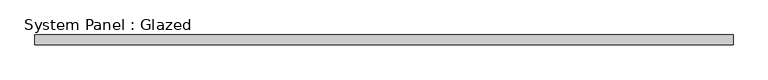
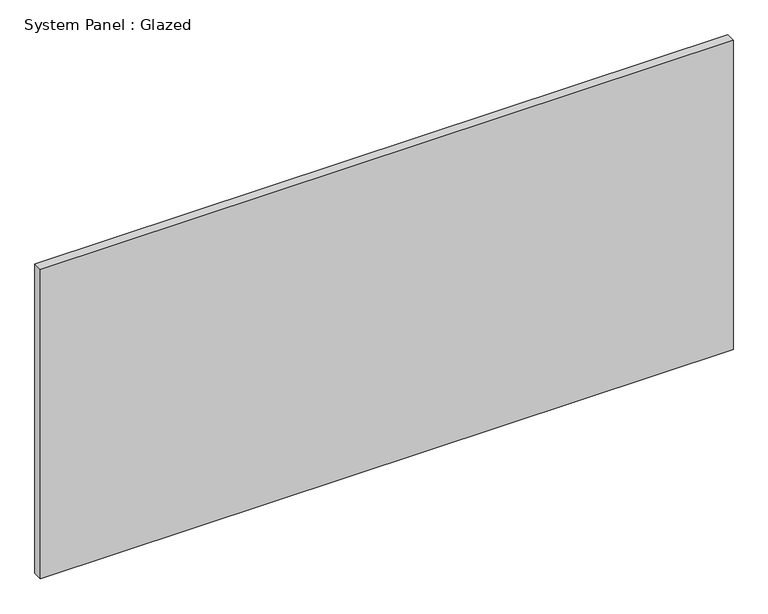
"""IFC4 building model written with IfcOpenShell, lengths in millimetres: plate geometry, System Panel : Glazed."""

from ifc_helpers import new_model, si_unit, origin, origin_with_axes, place, context, project, spatial, polyline, outline, extrude, source, transform, mapped, element, save


def system_panel_glazed_6b40402c(model_context):
    return source(origin(), model_context, "Body", "SweptSolid", [
        extrude(outline(polyline([(914.4, 19.05), (-914.4, 19.05), (-914.4, 44.45), (914.4, 44.45), (914.4, 19.05)])), origin_with_axes(), (0.0, 0.0, 1.0), 863.6),
    ])


if __name__ == "__main__":
    model = new_model("IFC4")
    model_context = context("Model", 3, world=origin())
    ifc_project = project(units=[si_unit("LENGTHUNIT", "METRE", prefix="MILLI")], contexts=[model_context])
    site = spatial("IfcSite", under=ifc_project)
    building = spatial("IfcBuilding", under=site)
    placement = place(None, origin())
    system_panel_glazed_shape = system_panel_glazed_6b40402c(model_context)
    element("IfcPlate", 1, ObjectType="System Panel : Glazed", at=placement, inside=building, context=model_context, shape_type="MappedRepresentation", body=[
        mapped(system_panel_glazed_shape, transform((0.0, 0.0, 0.0), x_axis=(1.0, 0.0, 0.0), y_axis=(0.0, 1.0, 0.0), z_axis=(0.0, 0.0, 1.0))),
    ])
    save(model, "model.ifc")

# Revit data of these elements
# Type "System Panel : Glazed"
#   Construction Type Id = "GSP4R"
#   Analytic Construction = "1/8 in Pilkington single glazing"
#   Visual Light Transmittance = 0.9
#   Solar Heat Gain Coefficient = 0.86
#   Heat Transfer Coefficient (U) = 1.18115 BTU/(h·ft²·°F)
# Element 1 (IfcPlate, "System Panel : Glazed")
#   Materials on its faces: "Glass"
# Materials
#   "Glass": class "Glass", colour RGB 0 128 192, transparency 0.75, Description = "Soda Lime Glass", Cost = 0
